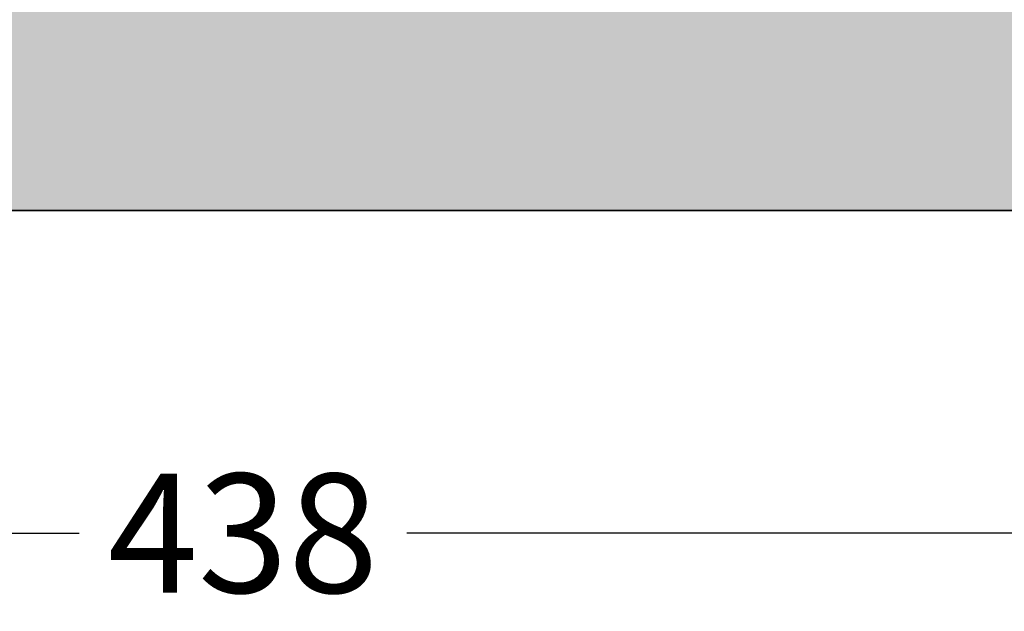
# Model space of a CAD drawing. Units: millimetres. Extents: x 130 to 1021, y 147 to 699.
# Tile 9 of 40: x 481 to 646, y 147 to 246. Entities that reach past the tile are written whole.
import ezdxf

# ---------------------------------------------------------------- set-up
doc = ezdxf.new("R2010")
doc.units = ezdxf.units.MM
doc.header["$MEASUREMENT"] = 0
for name, color, linetype, lineweight in [('A-ANNO-DIMS', 2, 'Continuous', 18), ('A-ELEV', 7, 'Continuous', 35), ('A-ELEV-PATT', 9, 'Continuous', 13)]:
    doc.layers.add(name, color=color, linetype=linetype, lineweight=lineweight)
doc.styles.get("Standard").update_dxf_attribs({"font": 'arial.ttf'})
doc.dimstyles.get("Standard").update_dxf_attribs({"dimtxt": 20, "dimasz": 10, "dimexe": 10, "dimexo": 10, "dimgap": 5, "dimtad": 0, "dimtih": 1, "dimtoh": 1, "dimdec": 0, "dimzin": 0, "dimdsep": 46, "dimtxsty": 'Standard', "dimcen": 5, "dimadec": 0, "dimazin": 0, "dimtfac": 1, "dimtdec": 0, "dimtofl": 0, "dimtmove": 0, "dimatfit": 3, "dimfxl": 1, "dimtolj": 1, "dimtzin": 0, "dimarcsym": 0})

# ---------------------------------------------------------------- blocks, each defined once
blk = doc.blocks.new('*D10')
at = {"layer": 'A-ANNO-DIMS', "color": 0, "lineweight": -2, "transparency": 16777216}
for p, q in [((440.89, 273.72), (430.89, 273.71)), ((473.57, 273.75), (483.57, 273.75)), ((450.9, 267.56), (450.9, 263.73)), ((463.58, 267.57), (463.58, 263.74))]:
    blk.add_line(p, q, dxfattribs=at)
at = {"layer": 'A-ANNO-DIMS', "color": 0, "transparency": 16777216}
for points in [[(440.89, 275.38), (440.89, 272.05), (450.89, 273.73)], [(473.57, 275.41), (473.58, 272.08), (463.57, 273.74)]]:
    blk.add_solid(points, dxfattribs=at)
at = {"layer": 'Defpoints', "color": 0, "transparency": 16777216}
for p in [(450.89, 277.56), (463.57, 277.57), (463.57, 273.74)]:
    blk.add_point(p, dxfattribs=at)
at = {"layer": 'A-ANNO-DIMS', "color": 0, "transparency": 16777216, "insert": (536.31, 273.75), "char_height": 20, "attachment_point": 5}
blk.add_mtext('\\A1;13 TYP.', dxfattribs=at)
blk = doc.blocks.new('*D11')
at = {"layer": 'A-ANNO-DIMS', "color": 0, "lineweight": -2, "transparency": 16777216}
for p, q in [((737.37, 648.7), (737.37, 149.74)), ((299.37, 566.95), (299.37, 149.74)), ((309.37, 159.74), (490.86, 159.74)), ((727.37, 159.74), (545.89, 159.74))]:
    blk.add_line(p, q, dxfattribs=at)
at = {"layer": 'A-ANNO-DIMS', "color": 0, "transparency": 16777216}
for points in [[(309.37, 161.41), (309.37, 158.07), (299.37, 159.74)], [(727.37, 161.41), (727.37, 158.07), (737.37, 159.74)]]:
    blk.add_solid(points, dxfattribs=at)
at = {"layer": 'Defpoints', "color": 0, "transparency": 16777216}
for p in [(737.37, 658.7), (299.37, 576.95), (737.37, 159.74)]:
    blk.add_point(p, dxfattribs=at)
at = {"layer": 'A-ANNO-DIMS', "color": 0, "transparency": 16777216, "insert": (518.37, 159.74), "char_height": 20, "attachment_point": 5}
blk.add_mtext('\\A1;438', dxfattribs=at)
blk = doc.blocks.new('*D12')
at = {"layer": 'A-ANNO-DIMS', "color": 0, "lineweight": -2, "transparency": 16777216}
for p, q in [((477.37, 661.95), (265.07, 661.95)), ((275.07, 651.95), (275.07, 438.2)), ((275.07, 194.04), (275.07, 407.78)), ((357.16, 184.04), (265.07, 184.04))]:
    blk.add_line(p, q, dxfattribs=at)
at = {"layer": 'A-ANNO-DIMS', "color": 0, "transparency": 16777216}
for points in [[(273.41, 651.95), (276.74, 651.95), (275.07, 661.95)], [(273.41, 194.04), (276.74, 194.04), (275.07, 184.04)]]:
    blk.add_solid(points, dxfattribs=at)
at = {"layer": 'Defpoints', "color": 0, "transparency": 16777216}
for p in [(275.07, 661.95), (487.37, 661.95), (367.16, 184.04)]:
    blk.add_point(p, dxfattribs=at)
at = {"layer": 'A-ANNO-DIMS', "color": 0, "transparency": 16777216, "insert": (275.07, 422.99), "char_height": 20, "attachment_point": 5}
blk.add_mtext('\\A1;477.9', dxfattribs=at)
blk = doc.blocks.new('*D23')
at = {"layer": 'A-ANNO-DIMS', "color": 0, "lineweight": -2, "transparency": 16777216}
for p, q in [((466.77, 403.95), (466.77, 696.25)), ((475.99, 209.04), (475.99, 696.25)), ((456.77, 686.25), (446.77, 686.25)), ((485.99, 686.25), (495.99, 686.25))]:
    blk.add_line(p, q, dxfattribs=at)
at = {"layer": 'A-ANNO-DIMS', "color": 0, "transparency": 16777216}
for points in [[(456.77, 687.91), (456.77, 684.58), (466.77, 686.25)], [(485.99, 687.91), (485.99, 684.58), (475.99, 686.25)]]:
    blk.add_solid(points, dxfattribs=at)
at = {"layer": 'Defpoints', "color": 0, "transparency": 16777216}
for p in [(475.99, 686.25), (466.77, 393.95), (475.99, 199.04)]:
    blk.add_point(p, dxfattribs=at)
at = {"layer": 'A-ANNO-DIMS', "color": 0, "transparency": 16777216, "insert": (534.63, 686.25), "char_height": 20, "attachment_point": 5}
blk.add_mtext('\\A1;9.222', dxfattribs=at)
blk = doc.blocks.new('*D24')
at = {"layer": 'A-ANNO-DIMS', "color": 0, "lineweight": -2, "transparency": 16777216}
for p, q in [((475.99, 209.04), (475.99, 696.25)), ((487.37, 671.95), (487.37, 696.25)), ((465.99, 686.25), (455.99, 686.25)), ((497.37, 686.25), (507.37, 686.25))]:
    blk.add_line(p, q, dxfattribs=at)
at = {"layer": 'A-ANNO-DIMS', "color": 0, "transparency": 16777216}
for points in [[(465.99, 687.91), (465.99, 684.58), (475.99, 686.25)], [(497.37, 687.91), (497.37, 684.58), (487.37, 686.25)]]:
    blk.add_solid(points, dxfattribs=at)
at = {"layer": 'Defpoints', "color": 0, "transparency": 16777216}
for p in [(487.37, 686.25), (487.37, 661.95), (475.99, 199.04)]:
    blk.add_point(p, dxfattribs=at)
at = {"layer": 'A-ANNO-DIMS', "color": 0, "transparency": 16777216, "insert": (553.02, 686.25), "char_height": 20, "attachment_point": 5}
blk.add_mtext('\\A1;11.385', dxfattribs=at)
blk = doc.blocks.new('*D49')
at = {"layer": 'A-ANNO-DIMS', "color": 0, "lineweight": -2, "transparency": 16777216}
for p, q in [((761.67, 283.95), (761.67, 293.95)), ((642.82, 273.95), (771.67, 273.95)), ((742.37, 213.95), (771.67, 213.95)), ((761.67, 203.95), (761.67, 193.95))]:
    blk.add_line(p, q, dxfattribs=at)
at = {"layer": 'A-ANNO-DIMS', "color": 0, "transparency": 16777216}
for points in [[(760.01, 283.95), (763.34, 283.95), (761.67, 273.95)], [(760.01, 203.95), (763.34, 203.95), (761.67, 213.95)]]:
    blk.add_solid(points, dxfattribs=at)
at = {"layer": 'Defpoints', "color": 0, "transparency": 16777216}
for p in [(632.82, 273.95), (761.67, 273.95), (732.37, 213.95)]:
    blk.add_point(p, dxfattribs=at)
at = {"layer": 'A-ANNO-DIMS', "color": 0, "transparency": 16777216, "insert": (761.67, 243.95), "char_height": 20, "attachment_point": 5}
blk.add_mtext('\\A1;60', dxfattribs=at)

msp = doc.modelspace()

# ---------------------------------------------------------------- hatches: boundary and pattern name
at = {"layer": 'A-ELEV-PATT'}
h = msp.add_hatch(color=256, dxfattribs=at)
h.dxf.hatch_style = 1
h.paths.add_polyline_path([(737.3738, 658.6988, 0.01359606), (632.4019, 661.9473), (607.3738, 661.9473), (487.3738, 661.9473), (487.3738, 649.9473), (607.3738, 649.9473), (632.3794, 649.9473, -0.01368411), (737.3738, 646.6784)])
h.paths.add_polyline_path([(732.3738, 643.9599, 0.01305286), (632.3738, 646.9473), (607.3738, 646.9473), (487.3738, 646.9473), (487.3738, 596.9473), (632.3738, 596.9473, -0.01305286), (732.3738, 593.9599)])
h.paths.add_polyline_path([(737.3738, 593.6732, 0.01370629), (632.3738, 596.9473), (487.3738, 596.9473), (487.3738, 586.9473), (632.355, 586.9473, -0.01378075), (737.3738, 583.6559)])
h.paths.add_polyline_path([(447.3738, 646.9473), (307.3738, 646.9473), (302.3738, 646.9473), (302.3738, 634.9473), (447.3738, 634.9473)])
h.paths.add_polyline_path([(447.3738, 631.9473), (307.3738, 631.9473), (307.3738, 586.9473), (447.3738, 586.9473)])
h.paths.add_polyline_path([(447.3738, 586.9473), (307.3738, 586.9473), (302.3738, 586.9473), (302.3738, 576.9473), (447.3738, 576.9473)])
h.paths.add_polyline_path([(447.3738, 573.9473), (367.3738, 573.9473), (367.3738, 539.9473), (447.3738, 539.9473)])
h.paths.add_polyline_path([(447.3738, 537.9473), (367.3738, 537.9473), (367.3738, 507.9473), (400.392, 507.4253, -0.00172798), (401.3281, 507.6451, -0.52200255), (425.6117, 511.0391, -0.03918489), (447.3738, 510.4359), (447.3738, 510.7883)])
h.paths.add_polyline_path([(394.7238, 505.9473), (367.3738, 505.9473), (367.3738, 476.9473, -0.0146512), (375.8501, 480.2159), (376.1506, 499.2266, -0.03554194)])
h.paths.add_polyline_path([(632.3738, 583.9473), (552.3738, 583.9473), (552.3738, 550.9473), (632.3738, 550.9473)])
h.paths.add_polyline_path([(632.3738, 548.9473), (552.3738, 548.9473), (552.3738, 515.9473), (632.3738, 515.9473)])
h.paths.add_polyline_path([(632.3738, 513.9473), (552.3738, 513.9473), (552.3738, 476.9473), (632.3738, 476.9473)])
h.paths.add_polyline_path([(737.3738, 473.6903, 0.01363261), (632.3926, 476.9473), (552.3738, 476.9473), (487.3738, 476.9473), (487.3738, 466.9473), (632.3738, 466.9473, -0.01370629), (737.3738, 463.6732)])
h.paths.add_polyline_path([(732.3738, 460.9552, 0.01307409), (632.3681, 463.9473), (487.3738, 463.9473), (487.3738, 407.735, -0.00322862), (489.3544, 406.9473), (632.3926, 406.9473, -0.01298259), (732.3738, 403.9755)])
h.paths.add_polyline_path([(487.3738, 463.9473, 0.20132998), (367.3738, 463.9473), (367.3738, 407.735, -0.18820307), (487.3738, 407.735)])
h.paths.add_polyline_path([(367.3738, 476.9473), (367.3738, 466.9473, -0.20133085), (487.3738, 466.9473), (487.3738, 476.9473, 0.20132998)])
h.paths.add_polyline_path([(367.3738, 463.9473), (307.3738, 463.9473), (307.3738, 401.9473), (357.9413, 401.9473), (367.3738, 407.735)])
h.paths.add_polyline_path([(367.3738, 476.9473), (302.3738, 476.9473), (302.3738, 466.9473), (367.3738, 466.9473)])
h.paths.add_polyline_path([(632.8184, 366.9453), (552.3738, 366.9453), (552.3738, 393.9473), (632.8184, 393.9473)])
h.paths.add_polyline_path([(632.8184, 357.2114), (632.8184, 363.9453), (552.3738, 363.9453), (552.3738, 357.2114), (552.3738, 336.9453), (632.8184, 336.9453)])
h.paths.add_polyline_path([(632.8184, 333.9453), (552.3738, 333.9453), (552.3738, 306.9453), (632.8184, 306.9453)])
h.paths.add_polyline_path([(632.8184, 303.9453), (552.3738, 303.9453), (552.3738, 273.9473), (632.355, 273.9473, 0.00006077), (632.8184, 273.9491)])
h.paths.add_polyline_path([(737.3738, 403.6903, 0.01363261), (632.3926, 406.9473), (489.3544, 406.9473, 0.19154808), (367.3738, 407.735), (367.3738, 396.9473, -0.20133085), (487.3738, 396.9473), (632.3738, 396.9473, -0.01370629), (737.3738, 393.6732)])
h.paths.add_polyline_path([(357.9413, 401.9473), (307.3738, 401.9473), (307.3738, 391.9473), (357.9413, 391.9473)])
h.paths.add_polyline_path([(357.9413, 357.2114), (357.9413, 388.9473), (307.3738, 388.9473), (307.3738, 357.2114), (307.3738, 273.9473), (357.9413, 273.9473)])
h.paths.add_polyline_path([(732.3738, 263.93, -0.0130317), (632.3794, 260.9473), (466.7667, 260.9473), (466.7667, 240.9473), (469.8406, 236.978), (469.8406, 221.978), (472.9145, 218.0087), (472.9145, 213.9473), (607.3738, 213.9473), (732.3738, 213.9473)])
h.paths.add_polyline_path([(732.3738, 290.889), (722.479, 290.889), (722.479, 301.889), (732.3738, 301.889), (732.3738, 305.889), (722.479, 305.889), (722.479, 316.889), (732.3738, 316.889), (732.3738, 320.889), (722.479, 320.889), (722.479, 331.889), (732.3738, 331.889), (732.3738, 335.889), (722.479, 335.889), (722.479, 346.889), (732.3738, 346.889), (732.3738, 350.889), (722.479, 350.889), (722.479, 361.889), (732.3738, 361.889), (732.3738, 365.889), (722.479, 365.889), (722.479, 376.889), (732.3738, 376.889), (732.3738, 380.889), (722.479, 380.889), (722.479, 391.4848, 0.00052326), (718.479, 391.6843), (718.479, 380.889), (707.479, 380.889), (707.479, 392.1896, 0.00052307), (703.479, 392.3576), (703.479, 380.889), (692.479, 380.889), (692.479, 392.7765, 0.00052292), (688.479, 392.9131), (688.479, 380.889), (677.479, 380.889), (677.479, 393.2456, 0.00052279), (673.479, 393.3508), (673.479, 380.889), (662.479, 380.889), (662.479, 393.597, 0.0005227), (658.479, 393.6709), (658.479, 380.889), (647.479, 380.889), (647.479, 393.8308, 0.00052264), (643.479, 393.8732), (643.479, 380.889), (632.8184, 380.889), (632.8184, 376.889), (643.479, 376.889), (643.479, 365.889), (632.8184, 365.889), (632.8184, 361.889), (643.479, 361.889), (643.479, 350.889), (632.8184, 350.889), (632.8184, 346.889), (643.479, 346.889), (643.479, 335.889), (632.8184, 335.889), (632.8184, 331.889), (643.479, 331.889), (643.479, 320.889), (632.8184, 320.889), (632.8184, 316.889), (643.479, 316.889), (643.479, 305.889), (632.8184, 305.889), (632.8184, 301.889), (643.479, 301.889), (643.479, 290.889), (632.8184, 290.889), (632.8184, 286.889), (643.479, 286.889), (643.479, 274.0217, 0.00052456), (647.479, 274.0643), (647.479, 286.889), (658.479, 286.889), (658.479, 274.2248, 0.00052462), (662.479, 274.2989), (662.479, 286.889), (673.479, 286.889), (673.479, 274.546, 0.00052471), (677.479, 274.6516), (677.479, 286.889), (688.479, 286.889), (688.479, 274.9853, 0.00052484), (692.479, 275.1224), (692.479, 286.889), (703.479, 286.889), (703.479, 275.5429, 0.000525), (707.479, 275.7115), (707.479, 286.889), (718.479, 286.889), (718.479, 276.2187, 0.00052519), (722.479, 276.4189), (722.479, 286.889), (732.3738, 286.889)])
h.paths.add_polyline_path([(718.479, 290.889), (707.479, 290.889), (707.479, 301.889), (718.479, 301.889)], flags=16)
h.paths.add_polyline_path([(703.479, 290.889), (692.479, 290.889), (692.479, 301.889), (703.479, 301.889)], flags=16)
h.paths.add_polyline_path([(718.479, 305.889), (707.479, 305.889), (707.479, 316.889), (718.479, 316.889)], flags=16)
h.paths.add_polyline_path([(703.479, 305.889), (692.479, 305.889), (692.479, 316.889), (703.479, 316.889)], flags=16)
h.paths.add_polyline_path([(688.479, 290.889), (677.479, 290.889), (677.479, 301.889), (688.479, 301.889)], flags=16)
h.paths.add_polyline_path([(718.479, 320.889), (707.479, 320.889), (707.479, 331.889), (718.479, 331.889)], flags=16)
h.paths.add_polyline_path([(688.479, 305.889), (677.479, 305.889), (677.479, 316.889), (688.479, 316.889)], flags=16)
h.paths.add_polyline_path([(703.479, 320.889), (692.479, 320.889), (692.479, 331.889), (703.479, 331.889)], flags=16)
h.paths.add_polyline_path([(688.479, 320.889), (677.479, 320.889), (677.479, 331.889), (688.479, 331.889)], flags=16)
h.paths.add_polyline_path([(673.479, 290.889), (662.479, 290.889), (662.479, 301.889), (673.479, 301.889)], flags=16)
h.paths.add_polyline_path([(718.479, 335.889), (707.479, 335.889), (707.479, 346.889), (718.479, 346.889)], flags=16)
h.paths.add_polyline_path([(673.479, 305.889), (662.479, 305.889), (662.479, 316.889), (673.479, 316.889)], flags=16)
h.paths.add_polyline_path([(703.479, 335.889), (692.479, 335.889), (692.479, 346.889), (703.479, 346.889)], flags=16)
h.paths.add_polyline_path([(673.479, 320.889), (662.479, 320.889), (662.479, 331.889), (673.479, 331.889)], flags=16)
h.paths.add_polyline_path([(688.479, 335.889), (677.479, 335.889), (677.479, 346.889), (688.479, 346.889)], flags=16)
h.paths.add_polyline_path([(658.479, 290.889), (647.479, 290.889), (647.479, 301.889), (658.479, 301.889)], flags=16)
h.paths.add_polyline_path([(718.479, 350.889), (707.479, 350.889), (707.479, 361.889), (718.479, 361.889)], flags=16)
h.paths.add_polyline_path([(658.479, 305.889), (647.479, 305.889), (647.479, 316.889), (658.479, 316.889)], flags=16)
h.paths.add_polyline_path([(703.479, 350.889), (692.479, 350.889), (692.479, 361.889), (703.479, 361.889)], flags=16)
h.paths.add_polyline_path([(673.479, 335.889), (662.479, 335.889), (662.479, 346.889), (673.479, 346.889)], flags=16)
h.paths.add_polyline_path([(658.479, 320.889), (647.479, 320.889), (647.479, 331.889), (658.479, 331.889)], flags=16)
h.paths.add_polyline_path([(688.479, 350.889), (677.479, 350.889), (677.479, 361.889), (688.479, 361.889)], flags=16)
h.paths.add_polyline_path([(718.479, 365.889), (707.479, 365.889), (707.479, 376.889), (718.479, 376.889)], flags=16)
h.paths.add_polyline_path([(658.479, 335.889), (647.479, 335.889), (647.479, 346.889), (658.479, 346.889)], flags=16)
h.paths.add_polyline_path([(673.479, 350.889), (662.479, 350.889), (662.479, 361.889), (673.479, 361.889)], flags=16)
h.paths.add_polyline_path([(703.479, 365.889), (692.479, 365.889), (692.479, 376.889), (703.479, 376.889)], flags=16)
h.paths.add_polyline_path([(688.479, 365.889), (677.479, 365.889), (677.479, 376.889), (688.479, 376.889)], flags=16)
h.paths.add_polyline_path([(658.479, 350.889), (647.479, 350.889), (647.479, 361.889), (658.479, 361.889)], flags=16)
h.paths.add_polyline_path([(673.479, 365.889), (662.479, 365.889), (662.479, 376.889), (673.479, 376.889)], flags=16)
h.paths.add_polyline_path([(658.479, 365.889), (647.479, 365.889), (647.479, 376.889), (658.479, 376.889)], flags=16)
h.paths.add_polyline_path([(732.3738, 503.9786), (722.3392, 503.9786), (722.3392, 514.9786), (732.3738, 514.9786), (732.3738, 518.9786), (722.3392, 518.9786), (722.3392, 529.9786), (732.3738, 529.9786), (732.3738, 533.9786), (722.3392, 533.9786), (722.3392, 544.9786), (732.3738, 544.9786), (732.3738, 546.9473), (732.3738, 548.9786), (722.3392, 548.9786), (722.3392, 559.9786), (732.3738, 559.9786), (732.3738, 563.9786), (722.3392, 563.9786), (722.3392, 574.9786), (732.3738, 574.9786), (732.3738, 578.9786), (722.3392, 578.9786), (722.3392, 581.4789, 0.00052601), (718.3392, 581.6791), (718.3392, 578.9786), (707.3392, 578.9786), (707.3392, 582.1863, 0.00052582), (703.3392, 582.355), (703.3392, 578.9786), (692.3392, 578.9786), (692.3392, 582.7752, 0.00052566), (688.3392, 582.9123), (688.3392, 578.9786), (677.3392, 578.9786), (677.3392, 583.2457, 0.00052554), (673.3392, 583.3512), (673.3392, 578.9786), (662.3392, 578.9786), (662.3392, 583.5978, 0.00052545), (658.3392, 583.6718), (658.3392, 578.9786), (647.3392, 578.9786), (647.3392, 583.8317, 0.00052539), (643.3392, 583.8741), (643.3392, 578.9786), (632.3738, 578.9786), (632.3738, 574.9786), (643.3392, 574.9786), (643.3392, 563.9786), (632.3738, 563.9786), (632.3738, 559.9786), (643.3392, 559.9786), (643.3392, 548.9786), (632.3738, 548.9786), (632.3738, 544.9786), (643.3392, 544.9786), (643.3392, 533.9786), (632.3738, 533.9786), (632.3738, 529.9786), (643.3392, 529.9786), (643.3392, 518.9786), (632.3738, 518.9786), (632.3738, 515.9473), (632.3738, 514.9786), (643.3392, 514.9786), (643.3392, 503.9786), (632.3738, 503.9786), (632.3738, 499.9786), (643.3392, 499.9786), (643.3392, 488.9786), (632.3738, 488.9786), (632.3738, 484.9786), (643.3392, 484.9786), (643.3392, 476.8751, -0.00051911), (647.3392, 476.8332), (647.3392, 484.9786), (658.3392, 484.9786), (658.3392, 476.6752, -0.00051917), (662.3392, 476.6022), (662.3392, 484.9786), (673.3392, 484.9786), (673.3392, 476.3585, -0.00051926), (677.3392, 476.2543), (677.3392, 484.9786), (688.3392, 484.9786), (688.3392, 475.9248, -0.00051938), (692.3392, 475.7894), (692.3392, 484.9786), (703.3392, 484.9786), (703.3392, 475.3741, -0.00051953), (707.3392, 475.2075), (707.3392, 484.9786), (718.3392, 484.9786), (718.3392, 474.7064, -0.00051972), (722.3392, 474.5086), (722.3392, 484.9786), (732.3738, 484.9786), (732.3738, 488.9786), (722.3392, 488.9786), (722.3392, 499.9786), (732.3738, 499.9786)])
h.paths.add_polyline_path([(718.3392, 503.9786), (707.3392, 503.9786), (707.3392, 514.9786), (718.3392, 514.9786)], flags=16)
h.paths.add_polyline_path([(718.3392, 499.9786), (718.3392, 488.9786), (707.3392, 488.9786), (707.3392, 499.9786)], flags=16)
h.paths.add_polyline_path([(718.3392, 518.9786), (707.3392, 518.9786), (707.3392, 529.9786), (718.3392, 529.9786)], flags=16)
h.paths.add_polyline_path([(703.3392, 503.9786), (692.3392, 503.9786), (692.3392, 514.9786), (703.3392, 514.9786)], flags=16)
h.paths.add_polyline_path([(703.3392, 499.9786), (703.3392, 488.9786), (692.3392, 488.9786), (692.3392, 499.9786)], flags=16)
h.paths.add_polyline_path([(703.3392, 518.9786), (692.3392, 518.9786), (692.3392, 529.9786), (703.3392, 529.9786)], flags=16)
h.paths.add_polyline_path([(718.3392, 533.9786), (707.3392, 533.9786), (707.3392, 544.9786), (718.3392, 544.9786)], flags=16)
h.paths.add_polyline_path([(688.3392, 503.9786), (677.3392, 503.9786), (677.3392, 514.9786), (688.3392, 514.9786)], flags=16)
h.paths.add_polyline_path([(688.3392, 499.9786), (688.3392, 488.9786), (677.3392, 488.9786), (677.3392, 499.9786)], flags=16)
h.paths.add_polyline_path([(703.3392, 533.9786), (692.3392, 533.9786), (692.3392, 544.9786), (703.3392, 544.9786)], flags=16)
h.paths.add_polyline_path([(688.3392, 518.9786), (677.3392, 518.9786), (677.3392, 529.9786), (688.3392, 529.9786)], flags=16)
h.paths.add_polyline_path([(688.3392, 533.9786), (677.3392, 533.9786), (677.3392, 544.9786), (688.3392, 544.9786)], flags=16)
h.paths.add_polyline_path([(718.3392, 548.9786), (707.3392, 548.9786), (707.3392, 559.9786), (718.3392, 559.9786)], flags=16)
h.paths.add_polyline_path([(673.3392, 503.9786), (662.3392, 503.9786), (662.3392, 514.9786), (673.3392, 514.9786)], flags=16)
h.paths.add_polyline_path([(673.3392, 499.9786), (673.3392, 488.9786), (662.3392, 488.9786), (662.3392, 499.9786)], flags=16)
h.paths.add_polyline_path([(703.3392, 548.9786), (692.3392, 548.9786), (692.3392, 559.9786), (703.3392, 559.9786)], flags=16)
h.paths.add_polyline_path([(673.3392, 518.9786), (662.3392, 518.9786), (662.3392, 529.9786), (673.3392, 529.9786)], flags=16)
h.paths.add_polyline_path([(688.3392, 548.9786), (677.3392, 548.9786), (677.3392, 559.9786), (688.3392, 559.9786)], flags=16)
h.paths.add_polyline_path([(673.3392, 533.9786), (662.3392, 533.9786), (662.3392, 544.9786), (673.3392, 544.9786)], flags=16)
h.paths.add_polyline_path([(718.3392, 563.9786), (707.3392, 563.9786), (707.3392, 574.9786), (718.3392, 574.9786)], flags=16)
h.paths.add_polyline_path([(658.3392, 503.9786), (647.3392, 503.9786), (647.3392, 514.9786), (658.3392, 514.9786)], flags=16)
h.paths.add_polyline_path([(658.3392, 499.9786), (658.3392, 488.9786), (647.3392, 488.9786), (647.3392, 499.9786)], flags=16)
h.paths.add_polyline_path([(703.3392, 563.9786), (692.3392, 563.9786), (692.3392, 574.9786), (703.3392, 574.9786)], flags=16)
h.paths.add_polyline_path([(658.3392, 518.9786), (647.3392, 518.9786), (647.3392, 529.9786), (658.3392, 529.9786)], flags=16)
h.paths.add_polyline_path([(673.3392, 548.9786), (662.3392, 548.9786), (662.3392, 559.9786), (673.3392, 559.9786)], flags=16)
h.paths.add_polyline_path([(688.3392, 563.9786), (677.3392, 563.9786), (677.3392, 574.9786), (688.3392, 574.9786)], flags=16)
h.paths.add_polyline_path([(658.3392, 533.9786), (647.3392, 533.9786), (647.3392, 544.9786), (658.3392, 544.9786)], flags=16)
h.paths.add_polyline_path([(673.3392, 563.9786), (662.3392, 563.9786), (662.3392, 574.9786), (673.3392, 574.9786)], flags=16)
h.paths.add_polyline_path([(658.3392, 548.9786), (647.3392, 548.9786), (647.3392, 559.9786), (658.3392, 559.9786)], flags=16)
h.paths.add_polyline_path([(658.3392, 563.9786), (647.3392, 563.9786), (647.3392, 574.9786), (658.3392, 574.9786)], flags=16)

# ---------------------------------------------------------------- linework, layer by layer
at = {"layer": 'A-ELEV'}
for p, q in [((472.9145, 213.9473), (607.3738, 213.9473)), ((607.3738, 213.9473), (732.3738, 213.9473))]:
    msp.add_line(p, q, dxfattribs=at)

# ---------------------------------------------------------------- dimensions: what is measured, and where the dimension line sits
at = {"layer": 'A-ANNO-DIMS'}
for base, p1, p2, override, picture, middle in [((475.9885, 686.2473), (466.7667, 393.9473), (475.9885, 199.0395), {"dimdec": 3, "dimlfac": 1, "dimrnd": 0, "dimzin": 0, "dimdsep": 46, "dimlunit": 2}, '*D23', (534.631, 686.2473)), ((487.3738, 686.2473), (475.9885, 199.0395), (487.3738, 661.9473), {"dimdec": 3, "dimlfac": 1, "dimrnd": 0, "dimzin": 0, "dimdsep": 46, "dimlunit": 2}, '*D24', (553.0218, 686.2473)), ((737.3738, 159.7395), (299.3738, 576.9473), (737.3738, 658.6988), {"dimdec": 0, "dimlfac": 1, "dimrnd": 0, "dimzin": 0, "dimdsep": 46, "dimlunit": 2}, '*D11', (518.3738, 159.7395))]:
    dim = msp.add_linear_dim(base=base, p1=p1, p2=p2, dimstyle='Standard', override=override, dxfattribs=at)
    dim.commit()
    dim.dimension.update_dxf_attribs({"geometry": picture, "text_midpoint": middle})
for base, p1, p2, override, picture, middle in [((275.0738, 661.9473), (367.163, 184.0395), (487.3738, 661.9473), {"dimdec": 1, "dimlfac": 1, "dimrnd": 0, "dimzin": 0, "dimdsep": 46, "dimlunit": 2}, '*D12', (275.0738, 422.9934)), ((761.6738, 273.9473), (732.3738, 213.9473), (632.8184, 273.9473), {"dimdec": 0, "dimlfac": 1, "dimrnd": 0, "dimzin": 0, "dimdsep": 46, "dimlunit": 2}, '*D49', (761.6738, 243.9473))]:
    dim = msp.add_linear_dim(base=base, p1=p1, p2=p2, angle=90, dimstyle='Standard', override=override, dxfattribs=at)
    dim.commit()
    dim.dimension.update_dxf_attribs({"geometry": picture, "text_midpoint": middle})
dim = msp.add_linear_dim(base=(463.5746, 273.7371), p1=(450.8885, 277.5595), p2=(463.5714, 277.5701), angle=0.047753, text='<> TYP.', dimstyle='Standard', override={"dimdec": 0, "dimrnd": 0, "dimzin": 0, "dimlunit": 2}, dxfattribs=at)
dim.commit()
dim.dimension.update_dxf_attribs({"geometry": '*D10', "text_midpoint": (536.3099, 273.7537)})

doc.saveas('drawing.dxf')
